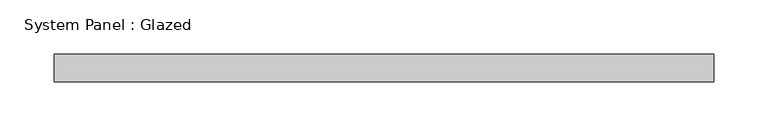
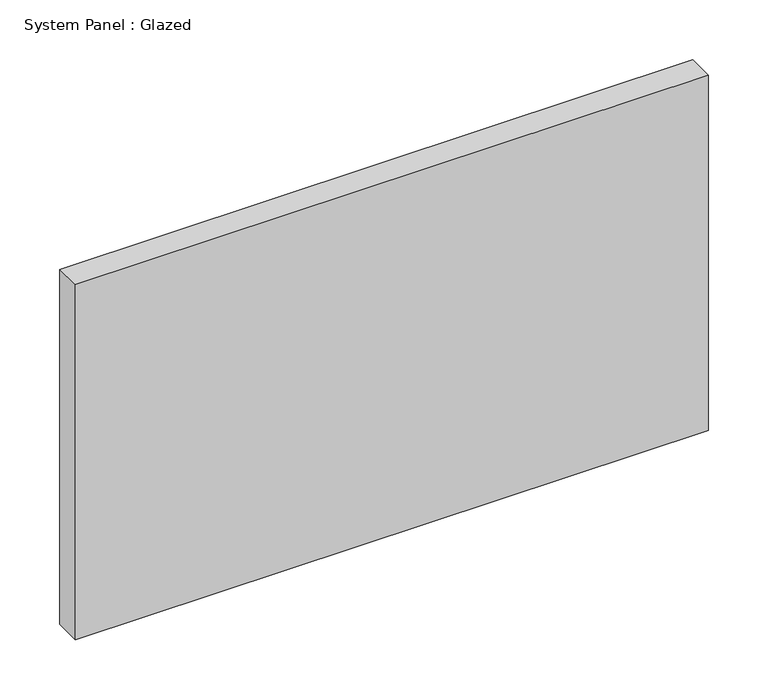
"""IFC4 building model written with IfcOpenShell, lengths in millimetres: plate geometry, System Panel : Glazed."""

from ifc_helpers import new_model, si_unit, origin, origin_with_axes, place, context, project, spatial, polyline, outline, extrude, source, transform, mapped, element, save


def system_panel_glazed_0920ec04(model_context):
    return source(origin(), model_context, "Body", "SweptSolid", [
        extrude(outline(polyline([(304.8, 19.05), (-304.8, 19.05), (-304.8, 44.45), (304.8, 44.45), (304.8, 19.05)])), origin_with_axes(), (0.0, 0.0, 1.0), 361.95),
    ])


if __name__ == "__main__":
    model = new_model("IFC4")
    model_context = context("Model", 3, world=origin())
    ifc_project = project(units=[si_unit("LENGTHUNIT", "METRE", prefix="MILLI")], contexts=[model_context])
    site = spatial("IfcSite", under=ifc_project)
    building = spatial("IfcBuilding", under=site)
    placement = place(None, origin())
    system_panel_glazed_shape = system_panel_glazed_0920ec04(model_context)
    element("IfcPlate", 1, ObjectType="System Panel : Glazed", at=placement, inside=building, context=model_context, shape_type="MappedRepresentation", body=[
        mapped(system_panel_glazed_shape, transform((0.0, 0.0, 0.0), x_axis=(1.0, 0.0, 0.0), y_axis=(0.0, 1.0, 0.0), z_axis=(0.0, 0.0, 1.0))),
    ])
    save(model, "model.ifc")

# Revit data of these elements
# Type "System Panel : Glazed"
#   Construction Type Id = "GSP4R"
#   Analytic Construction = "1/8 in Pilkington single glazing"
#   Visual Light Transmittance = 0.9
#   Solar Heat Gain Coefficient = 0.86
#   Heat Transfer Coefficient (U) = 1.18115 BTU/(h·ft²·°F)
#   Define Thermal Properties by = 1
# Element 1 (IfcPlate, "System Panel : Glazed")
#   Materials on its faces: "Glass"
# Materials
#   "Glass": class "Glass", colour RGB 0 128 192, transparency 0.75, Description = "Soda Lime Glass", Cost = 0
